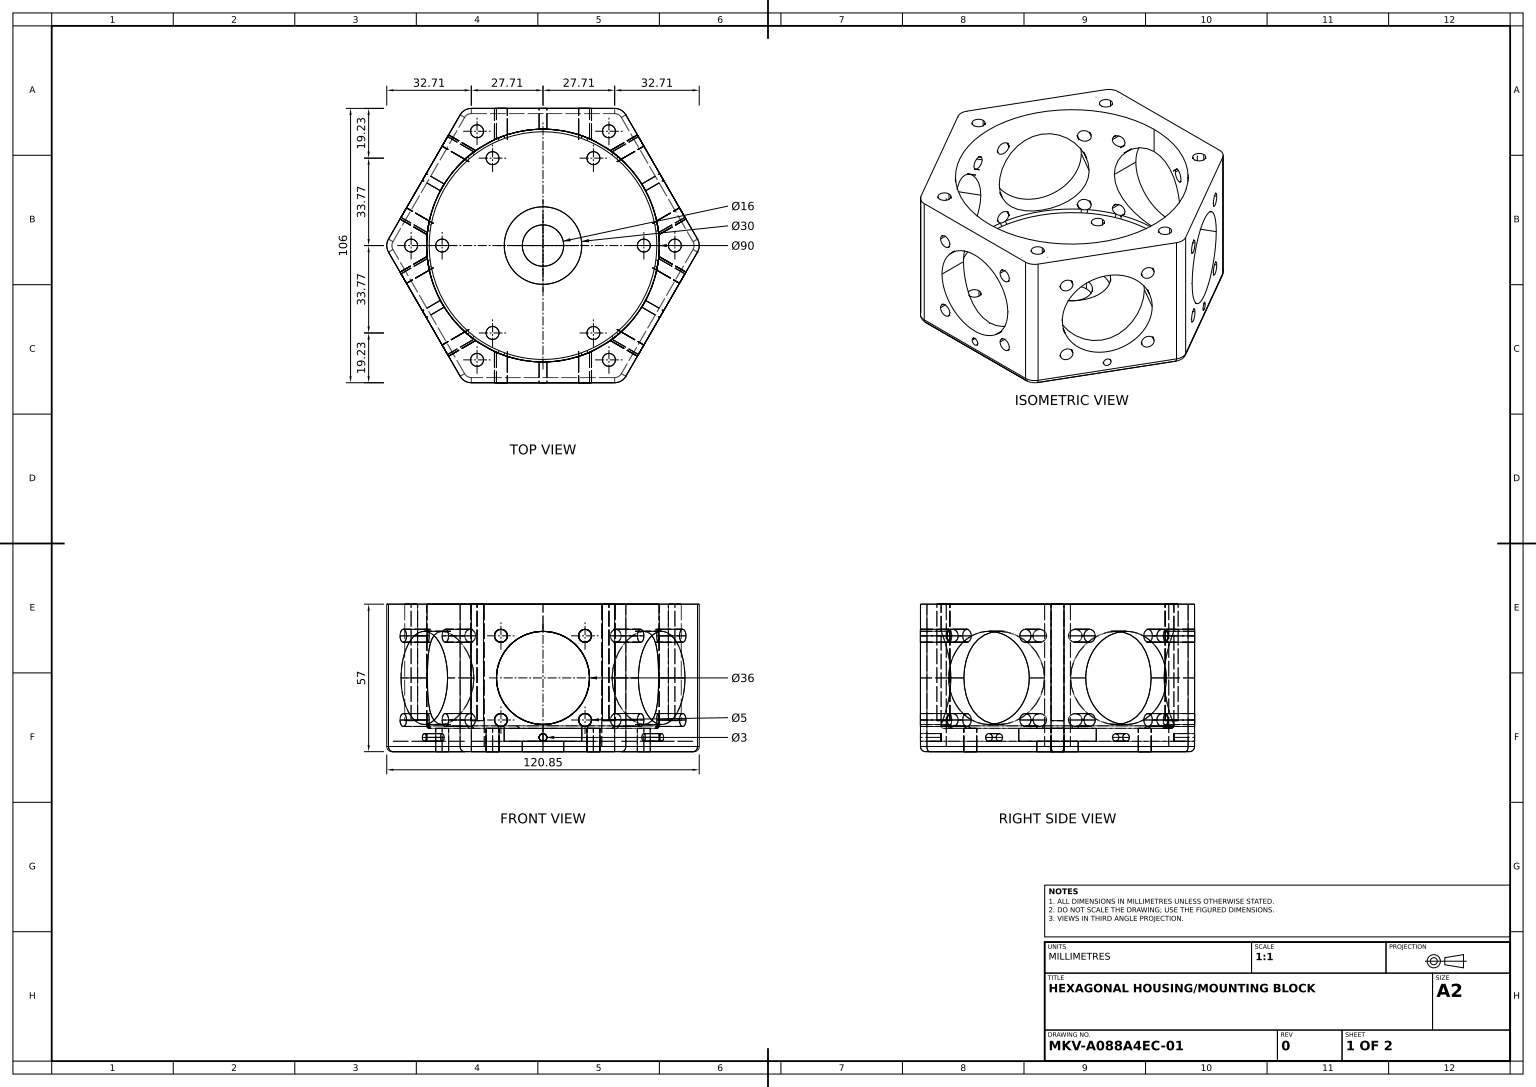
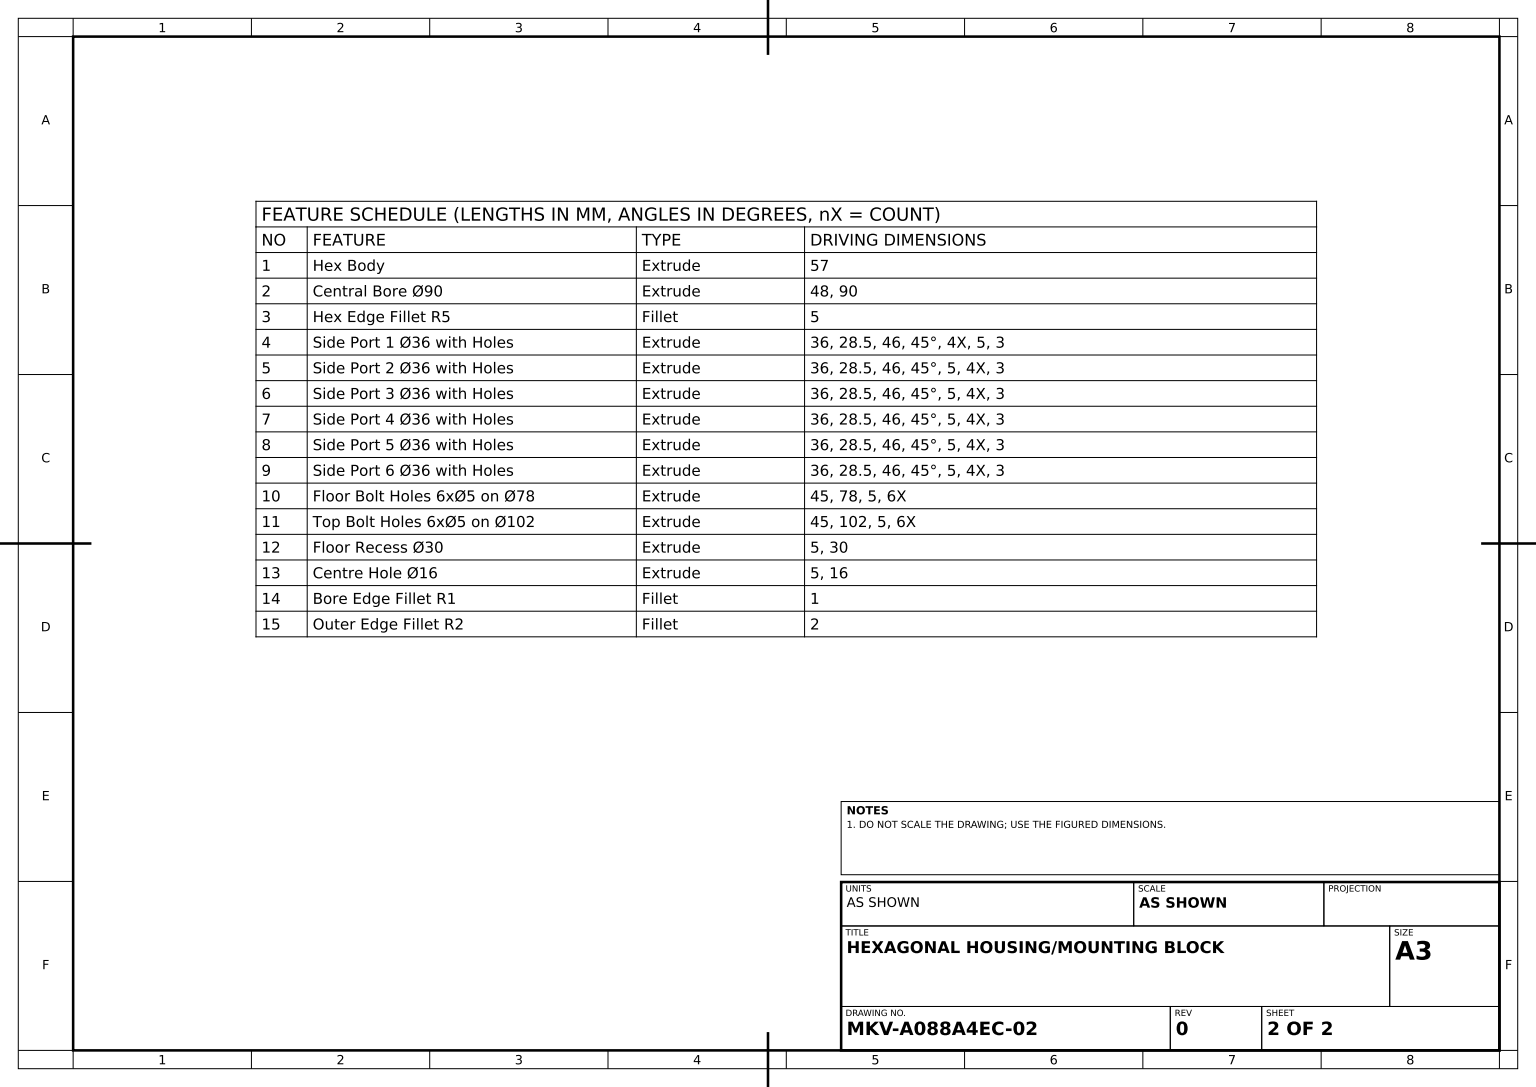
SolidWorks part; units mm, degrees
material "Plain Carbon Steel"
ref_plane "Front Plane" through (0, 0, 0) normal (0, 0, 1) x (1, 0, 0)
ref_plane "Top Plane" through (0, 0, 0) normal (0, 1, 0) x (1, 0, 0)
ref_plane "Right Plane" through (0, 0, 0) normal (1, 0, 0) x (0, 0, -1)
sketch "Hex Body Profile Sketch" plane through (0, 0, 0) normal (0, 1, 0) x (1, 0, 0)
  line L1 (61.1991, 0) -> (30.5996, 53)
  line L2 (30.5996, 53) -> (-30.5996, 53)
  line L3 (-30.5996, 53) -> (-61.1991, 0)
  line L4 (-61.1991, 0) -> (-30.5996, -53)
  line L5 (-30.5996, -53) -> (30.5996, -53)
  line L6 (30.5996, -53) -> (61.1991, 0)
  circle A0 centre (0, 0) radius 53 construction
  dimension "D1" = 106
extrude "Hex Body" add sketch "Hex Body Profile Sketch" along normal blind 57
sketch "Central Bore Sketch" plane through (0, 57, 0) normal (0, 1, 0) x (1, 0, 0)
  circle A0 centre (0, 0) radius 45
  dimension "D1" = 90
extrude "Central Bore Ø90" cut sketch "Central Bore Sketch" against normal blind 48
fillet "Hex Edge Fillet R5" radius 5 6 edges at (30.5996, 28.5, -53) (-30.5996, 28.5, -53) (61.1991, 28.5, 0) (30.5996, 28.5, 53) (-61.1991, 28.5, 0) (-30.5996, 28.5, 53)
sketch "Side Port 1 Sketch" plane through (0, 0, -53) normal (0, 0, -1) x (-1, 0, 0)
  line L0 (-27.7128, 0) -> (27.7128, 0) construction
  line L1 (0, 28.5) -> (18.3527, 46.8527) construction
  line L2 (0, 28.5) -> (18.3527, 10.1473) construction
  line L3 (0, 28.5) -> (-18.3527, 10.1473) construction
  line L4 (0, 28.5) -> (-18.3527, 46.8527) construction
  circle A0 centre (0, 28.5) radius 18
  circle A1 centre (0, 28.5) radius 23 construction
  circle A2 centre (16.2635, 44.7635) radius 2.5
  circle A3 centre (16.2635, 12.2365) radius 2.5
  circle A4 centre (-16.2635, 12.2365) radius 2.5
  circle A5 centre (-16.2635, 44.7635) radius 2.5
  circle A6 centre (0, 5.5) radius 1.5
  dimension "D1" = 36
  dimension "D3" = 46
  dimension "D6" = 5
  dimension "D8" = 3
  dimension "D2" = 28.5
  dimension "D4" = 45
  dimension "D5" = 4
  dimension "D7" = 4
extrude "Side Port 1 Ø36 with Holes" cut sketch "Side Port 1 Sketch" against normal up to surface (11.7568 mm away)
sketch "Side Port 2 Sketch" plane through (-45.8993, 0, -26.5) normal (-0.866, 0, -0.5) x (-0.5, 0, 0.866)
  line L0 (-27.7128, 0) -> (27.7128, 0) construction
  line L1 (0, 28.5) -> (22.0108, 50.5108) construction
  circle A0 centre (0, 28.5) radius 18
  circle A1 centre (0, 28.5) radius 23 construction
  circle A2 centre (16.2635, 44.7635) radius 2.5
  circle A3 centre (16.2635, 12.2365) radius 2.5
  circle A4 centre (-16.2635, 12.2365) radius 2.5
  circle A5 centre (-16.2635, 44.7635) radius 2.5
  circle A6 centre (0, 5.5) radius 1.5
  dimension "D1" = 36
  dimension "D3" = 46
  dimension "D5" = 5
  dimension "D7" = 3
  dimension "D2" = 28.5
  dimension "D4" = 45
  dimension "D6" = 4
extrude "Side Port 2 Ø36 with Holes" cut sketch "Side Port 2 Sketch" against normal up to surface (11.7568 mm away)
sketch "Side Port 3 Sketch" plane through (-45.8993, 0, 26.5) normal (-0.866, 0, 0.5) x (0.5, 0, 0.866)
  line L0 (0, 28.5) -> (20.6138, 49.1138) construction
  circle A0 centre (0, 28.5) radius 18
  circle A1 centre (0, 28.5) radius 23 construction
  circle A2 centre (16.2635, 44.7635) radius 2.5
  circle A3 centre (16.2635, 12.2365) radius 2.5
  circle A4 centre (-16.2635, 12.2365) radius 2.5
  circle A5 centre (-16.2635, 44.7635) radius 2.5
  circle A6 centre (0, 5.5) radius 1.5
  dimension "D1" = 36
  dimension "D3" = 46
  dimension "D5" = 5
  dimension "D6" = 4
  dimension "D7" = 3
  dimension "D2" = 28.5
  dimension "D4" = 45
extrude "Side Port 3 Ø36 with Holes" cut sketch "Side Port 3 Sketch" against normal up to surface (11.7568 mm away)
sketch "Side Port 4 Sketch" plane through (0, 0, 53) normal (0, 0, 1) x (1, 0, 0)
  line L0 (-27.7128, 0) -> (27.7128, 0) construction
  line L1 (0, 28.5) -> (19.868, 48.368) construction
  circle A0 centre (0, 28.5) radius 18
  circle A1 centre (0, 28.5) radius 23 construction
  circle A2 centre (16.2635, 44.7635) radius 2.5
  circle A3 centre (16.2635, 12.2365) radius 2.5
  circle A4 centre (-16.2635, 12.2365) radius 2.5
  circle A5 centre (-16.2635, 44.7635) radius 2.5
  circle A6 centre (0, 5.5) radius 1.5
  dimension "D1" = 36
  dimension "D3" = 46
  dimension "D5" = 5
  dimension "D7" = 3
  dimension "D2" = 28.5
  dimension "D4" = 45
  dimension "D6" = 4
extrude "Side Port 4 Ø36 with Holes" cut sketch "Side Port 4 Sketch" against normal up to surface (11.7568 mm away)
sketch "Side Port 5 Sketch" plane through (45.8993, 0, 26.5) normal (0.866, 0, 0.5) x (0.5, 0, -0.866)
  line L0 (-27.7128, 0) -> (27.7128, 0) construction
  line L1 (0, 28.5) -> (21.407, 49.907) construction
  circle A0 centre (0, 28.5) radius 18
  circle A1 centre (0, 28.5) radius 23 construction
  circle A2 centre (16.2635, 44.7635) radius 2.5
  circle A3 centre (16.2635, 12.2365) radius 2.5
  circle A4 centre (-16.2635, 12.2365) radius 2.5
  circle A5 centre (-16.2635, 44.7635) radius 2.5
  circle A6 centre (0, 5.5) radius 1.5
  dimension "D1" = 36
  dimension "D3" = 46
  dimension "D5" = 5
  dimension "D7" = 3
  dimension "D2" = 28.5
  dimension "D4" = 45
  dimension "D6" = 4
extrude "Side Port 5 Ø36 with Holes" cut sketch "Side Port 5 Sketch" against normal up to surface (11.7568 mm away)
sketch "Side Port 6 Sketch" plane through (45.8993, 0, -26.5) normal (0.866, 0, -0.5) x (-0.5, 0, -0.866)
  line L0 (-27.7128, 0) -> (27.7128, 0) construction
  line L1 (0, 28.5) -> (21.3036, 49.8036) construction
  circle A0 centre (0, 28.5) radius 18
  circle A1 centre (0, 28.5) radius 23 construction
  circle A2 centre (16.2635, 44.7635) radius 2.5
  circle A3 centre (16.2635, 12.2365) radius 2.5
  circle A4 centre (-16.2635, 12.2365) radius 2.5
  circle A5 centre (-16.2635, 44.7635) radius 2.5
  circle A6 centre (0, 5.5) radius 1.5
  dimension "D1" = 36
  dimension "D3" = 46
  dimension "D5" = 5
  dimension "D7" = 3
  dimension "D2" = 28.5
  dimension "D4" = 45
  dimension "D6" = 4
extrude "Side Port 6 Ø36 with Holes" cut sketch "Side Port 6 Sketch" against normal up to surface (11.7568 mm away)
sketch "Floor Bolt Circle Sketch" plane through (0, 9, 0) normal (0, 1, 0) x (1, 0, 0)
  circle A0 centre (0, 0) radius 39 construction
  circle A1 centre (39, 0) radius 2.5
  circle A2 centre (19.5, -33.775) radius 2.5
  circle A3 centre (-19.5, -33.775) radius 2.5
  circle A4 centre (-39, 0) radius 2.5
  circle A5 centre (-19.5, 33.775) radius 2.5
  circle A6 centre (19.5, 33.775) radius 2.5
  dimension "D1" = 78
  dimension "D2" = 5
  dimension "D3" = 6
extrude "Floor Bolt Holes 6xØ5 on Ø78" cut sketch "Floor Bolt Circle Sketch" against normal blind 45
sketch "Top Bolt Circle Sketch" plane through (0, 57, 0) normal (0, 1, 0) x (1, 0, 0)
  circle A0 centre (0, 0) radius 51 construction
  circle A1 centre (51, 0) radius 2.5
  circle A2 centre (25.5, -44.1673) radius 2.5
  circle A3 centre (-25.5, -44.1673) radius 2.5
  circle A4 centre (-51, 0) radius 2.5
  circle A5 centre (-25.5, 44.1673) radius 2.5
  circle A6 centre (25.5, 44.1673) radius 2.5
  dimension "D1" = 102
  dimension "D2" = 5
  dimension "D3" = 6
extrude "Top Bolt Holes 6xØ5 on Ø102" cut sketch "Top Bolt Circle Sketch" against normal blind 45
sketch "Floor Recess Sketch" plane through (0, 9, 0) normal (0, 1, 0) x (1, 0, 0)
  circle A0 centre (0, 0) radius 15
  dimension "D1" = 30
extrude "Floor Recess Ø30" cut sketch "Floor Recess Sketch" against normal blind 5
sketch "Centre Hole Sketch" plane through (0, 4, 0) normal (0, 1, 0) x (1, 0, 0)
  circle A0 centre (0, 0) radius 8
  dimension "D1" = 16
extrude "Centre Hole Ø16" cut sketch "Centre Hole Sketch" against normal blind 5
fillet "Bore Edge Fillet R1" radius 1 1 edges at (0, 9, 45)
fillet "Outer Edge Fillet R2" radius 2 12 edges at (-30.2128, 0, 52.3301) (-45.8993, 0, 26.5) (-60.4256, 0, 0) (-45.8993, 0, -26.5) (-30.2128, 0, -52.3301) (0, 0, -53) (30.2128, 0, -52.3301) (45.8993, 0, -26.5) (60.4256, 0, 0) (45.8993, 0, 26.5) (30.2128, 0, 52.3301) (0, 0, 53)
